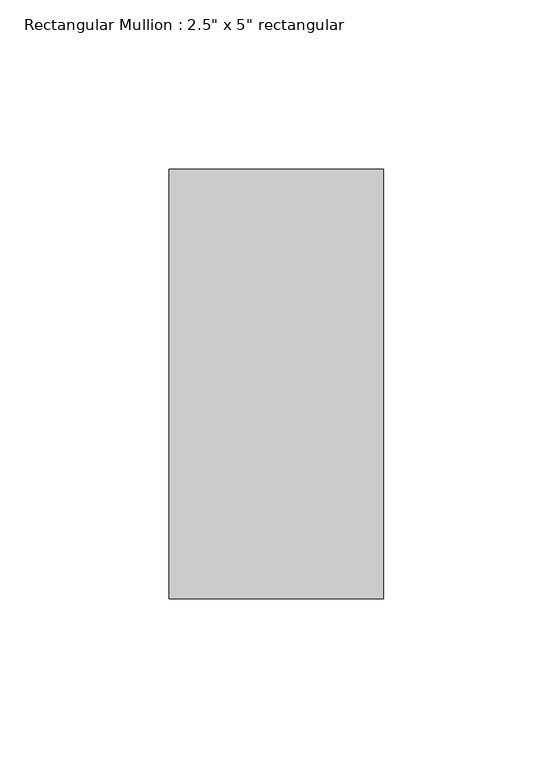
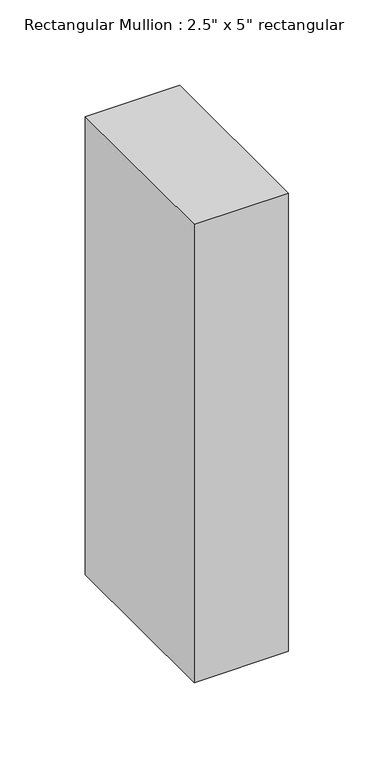
"""IFC4 building model written with IfcOpenShell, lengths in millimetres: member geometry."""

from ifc_helpers import new_model, si_unit, frame, origin, place, context, project, spatial, polyline, outline, extrude, source, transform, mapped, element, save


def member_2891061c(model_context):
    return source(origin(), model_context, "Body", "SweptSolid", [
        extrude(outline(polyline([(0.0, 63.5), (0.0, -63.5), (-63.5, -63.5), (-63.5, 63.5), (0.0, 63.5)])), frame((0.0, 0.0, -327.025), z_axis=(0.0, 0.0, 1.0), x_axis=(1.0, 0.0, 0.0)), (0.0, 0.0, 1.0), 327.025),
    ])


if __name__ == "__main__":
    model = new_model("IFC4")
    model_context = context("Model", 3, world=origin())
    ifc_project = project(units=[si_unit("LENGTHUNIT", "METRE", prefix="MILLI")], contexts=[model_context])
    site = spatial("IfcSite", under=ifc_project)
    building = spatial("IfcBuilding", under=site)
    placement = place(None, origin())
    member_shape = member_2891061c(model_context)
    element("IfcMember", 1, ObjectType="Rectangular Mullion : 2.5\" x 5\" rectangular", at=placement, inside=building, context=model_context, shape_type="MappedRepresentation", body=[
        mapped(member_shape, transform((0.0, 0.0, 0.0), x_axis=(1.0, 0.0, 0.0), y_axis=(0.0, 1.0, 0.0), z_axis=(0.0, 0.0, 1.0))),
    ])
    save(model, "model.ifc")

# Revit data of these elements
# Type "Rectangular Mullion : 2.5\" x 5\" rectangular"
#   built-in parameter 1007304 = 0.416667 (stored number, unit not read)
#   built-in parameter 1007301 = 0.104167 (stored number, unit not read)
#   built-in parameter 1007300 = 0.104167 (stored number, unit not read)
# Element 1 (IfcMember, "Rectangular Mullion : 2.5\" x 5\" rectangular")
#   Materials on its faces: "Aluminum"
# Materials
#   "Aluminum": class "Metal", colour RGB 247 247 247, transparency 0, Description = "Aluminum 6061", Cost = 0
